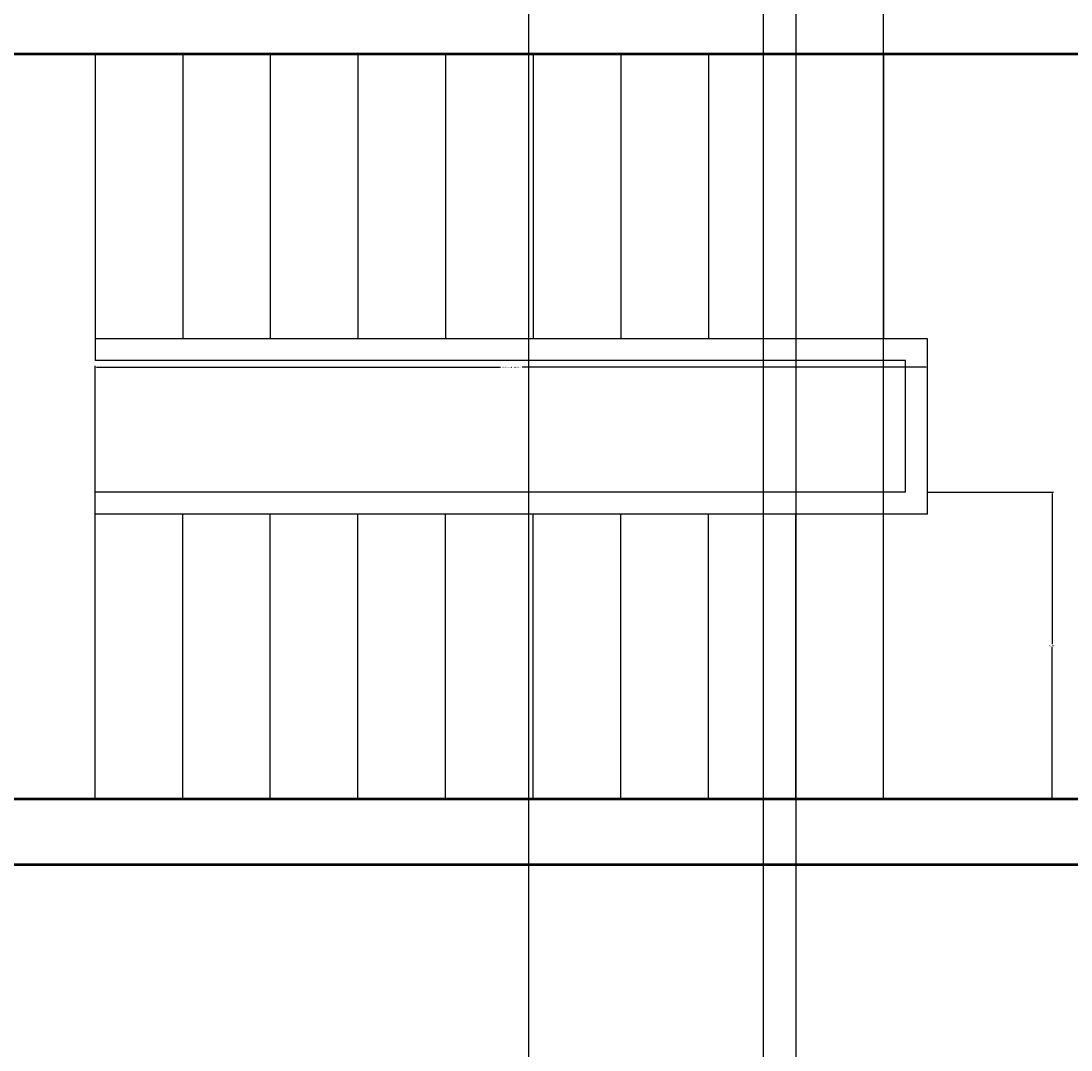
# Model space of a CAD drawing. Units: inches. Extents: x 5375 to 6084, y 16106 to 17259.
# Tile 13 of 32: x 5844 to 5988, y 16377 to 16518. Entities that reach past the tile are written whole.
import ezdxf

# ---------------------------------------------------------------- set-up
doc = ezdxf.new("R2010")
doc.units = ezdxf.units.IN
for name, color, linetype, lineweight in [('A-ANNO-DIMS', 2, 'Continuous', 18), ('STAIRCASE', 7, 'Continuous', 25), ('WALL', 6, 'Continuous', 50)]:
    doc.layers.add(name, color=color, linetype=linetype, lineweight=lineweight)
doc.styles.get("Standard").update_dxf_attribs({"font": 'arial.ttf'})
doc.dimstyles.get("Standard").update_dxf_attribs({"dimtxt": 0.18, "dimasz": 0.18, "dimexe": 0.18, "dimexo": 0.0625, "dimgap": 0.09, "dimtad": 0, "dimtih": 1, "dimtoh": 1, "dimdec": 4, "dimzin": 0, "dimdsep": 46, "dimtxsty": 'Standard', "dimcen": 0.09, "dimadec": 0, "dimazin": 0, "dimtfac": 1, "dimtdec": 4, "dimtofl": 0, "dimtmove": 0, "dimatfit": 3, "dimfxl": 1, "dimtolj": 1, "dimtzin": 0, "dimarcsym": 0})

# ---------------------------------------------------------------- blocks, each defined once
blk = doc.blocks.new('STAIR-FLIGHT-12IN-GOING')
for p, q in [((0, 42), (0, 0)), ((12, 42), (12, 3)), ((12, 42), (12, 3)), ((24, 42), (24, 3)), ((36, 42), (36, 3)), ((48, 42), (48, 3)), ((60, 42), (60, 3)), ((72, 42), (72, 3)), ((84, 42), (84, 3)), ((96, 42), (96, 3)), ((108, 42), (108, 3)), ((114, 3), (0, 3)), ((111, 0), (0, 0))]:
    blk.add_line(p, q)
blk = doc.blocks.new('*D24')
at = {"layer": 'A-ANNO-DIMS', "color": 0, "lineweight": -2, "transparency": 16777216}
for p, q in [((5854.62, 16453.64), (5854.62, 16470.86)), ((5854.8, 16470.68), (5910.14, 16470.68)), ((5968.44, 16470.68), (5913.1, 16470.68)), ((5968.62, 16453.64), (5968.62, 16470.86))]:
    blk.add_line(p, q, dxfattribs=at)
at = {"layer": 'A-ANNO-DIMS', "color": 0, "transparency": 16777216}
for points in [[(5854.8, 16470.71), (5854.8, 16470.65), (5854.62, 16470.68)], [(5968.44, 16470.71), (5968.44, 16470.65), (5968.62, 16470.68)]]:
    blk.add_solid(points, dxfattribs=at)
at = {"layer": 'Defpoints', "color": 0, "transparency": 16777216}
for p in [(5968.62, 16470.68), (5854.62, 16453.58), (5968.62, 16453.58)]:
    blk.add_point(p, dxfattribs=at)
at = {"layer": 'A-ANNO-DIMS', "color": 0, "transparency": 16777216, "insert": (5911.62, 16470.68), "char_height": 0.18, "attachment_point": 5}
blk.add_mtext('\\A1;STAIR FLIGHT 114 TYP.', dxfattribs=at)
blk = doc.blocks.new('*D25')
at = {"layer": 'A-ANNO-DIMS', "color": 0, "lineweight": -2, "transparency": 16777216}
for p, q in [((5968.68, 16453.58), (5985.9, 16453.58)), ((5985.72, 16453.4), (5985.72, 16432.76)), ((5985.72, 16411.76), (5985.72, 16432.4)), ((5968.68, 16411.58), (5985.9, 16411.58))]:
    blk.add_line(p, q, dxfattribs=at)
at = {"layer": 'A-ANNO-DIMS', "color": 0, "transparency": 16777216}
for points in [[(5985.69, 16453.4), (5985.75, 16453.4), (5985.72, 16453.58)], [(5985.69, 16411.76), (5985.75, 16411.76), (5985.72, 16411.58)]]:
    blk.add_solid(points, dxfattribs=at)
at = {"layer": 'Defpoints', "color": 0, "transparency": 16777216}
for p in [(5968.62, 16453.58), (5968.62, 16411.58), (5985.72, 16411.58)]:
    blk.add_point(p, dxfattribs=at)
at = {"layer": 'A-ANNO-DIMS', "color": 0, "transparency": 16777216, "insert": (5985.72, 16432.58), "char_height": 0.18, "attachment_point": 5}
blk.add_mtext('\\A1;42 TYP.', dxfattribs=at)
blk = doc.blocks.new('*D44')
at = {"layer": 'A-ANNO-DIMS', "color": 0, "lineweight": -2, "transparency": 16777216}
for p, q in [((5914, 16886.53), (5914, 16106.48)), ((5946.12, 16886.53), (5946.12, 16106.48)), ((5914.18, 16106.66), (5929.6, 16106.66)), ((5945.94, 16106.66), (5930.53, 16106.66))]:
    blk.add_line(p, q, dxfattribs=at)
at = {"layer": 'A-ANNO-DIMS', "color": 0, "transparency": 16777216}
for points in [[(5914.18, 16106.69), (5914.18, 16106.63), (5914, 16106.66)], [(5945.94, 16106.69), (5945.94, 16106.63), (5946.12, 16106.66)]]:
    blk.add_solid(points, dxfattribs=at)
at = {"layer": 'Defpoints', "color": 0, "transparency": 16777216}
for p in [(5914, 16886.6), (5946.12, 16886.6), (5914, 16106.66)]:
    blk.add_point(p, dxfattribs=at)
at = {"layer": 'A-ANNO-DIMS', "color": 0, "transparency": 16777216, "insert": (5930.06, 16106.66), "char_height": 0.18, "attachment_point": 5}
blk.add_mtext('\\A1;32.117', dxfattribs=at)
blk = doc.blocks.new('*D46')
at = {"layer": 'A-ANNO-DIMS', "color": 0, "lineweight": -2, "transparency": 16777216}
for p, q in [((5946.12, 16771.52), (5946.12, 16106.48)), ((5950.62, 16771.52), (5950.62, 16106.48)), ((5946.3, 16106.66), (5948.11, 16106.66)), ((5950.44, 16106.66), (5948.63, 16106.66))]:
    blk.add_line(p, q, dxfattribs=at)
at = {"layer": 'A-ANNO-DIMS', "color": 0, "transparency": 16777216}
for points in [[(5946.3, 16106.69), (5946.3, 16106.63), (5946.12, 16106.66)], [(5950.44, 16106.69), (5950.44, 16106.63), (5950.62, 16106.66)]]:
    blk.add_solid(points, dxfattribs=at)
at = {"layer": 'Defpoints', "color": 0, "transparency": 16777216}
for p in [(5946.12, 16771.58), (5950.62, 16771.58), (5950.62, 16106.66)]:
    blk.add_point(p, dxfattribs=at)
at = {"layer": 'A-ANNO-DIMS', "color": 0, "transparency": 16777216, "insert": (5948.37, 16106.66), "char_height": 0.18, "attachment_point": 5}
blk.add_mtext('\\A1;4.5', dxfattribs=at)
blk = doc.blocks.new('*D48')
at = {"layer": 'A-ANNO-DIMS', "color": 0, "lineweight": -2, "transparency": 16777216}
for p, q in [((5962.62, 16411.64), (5962.62, 17259.16)), ((5962.8, 17258.98), (5992.4, 17258.98)), ((6022.44, 17258.98), (5992.84, 17258.98)), ((6022.62, 16411.64), (6022.62, 17259.16))]:
    blk.add_line(p, q, dxfattribs=at)
at = {"layer": 'A-ANNO-DIMS', "color": 0, "transparency": 16777216}
for points in [[(5962.8, 17259.01), (5962.8, 17258.95), (5962.62, 17258.98)], [(6022.44, 17259.01), (6022.44, 17258.95), (6022.62, 17258.98)]]:
    blk.add_solid(points, dxfattribs=at)
at = {"layer": 'Defpoints', "color": 0, "transparency": 16777216}
for p in [(6022.62, 17258.98), (5962.62, 16411.58), (6022.62, 16411.58)]:
    blk.add_point(p, dxfattribs=at)
at = {"layer": 'A-ANNO-DIMS', "color": 0, "transparency": 16777216, "insert": (5992.62, 17258.98), "char_height": 0.18, "attachment_point": 5}
blk.add_mtext('\\A1;60', dxfattribs=at)

msp = doc.modelspace()

# ---------------------------------------------------------------- linework, layer by layer
at = {"layer": 'STAIRCASE'}
for p, q in [((5968.6199, 16450.5793), (5968.6199, 16474.5793)), ((5965.6199, 16453.5793), (5965.6199, 16471.5793))]:
    msp.add_line(p, q, dxfattribs=at)
at = {"layer": 'WALL'}
for p, q in [((5791.6199, 16513.5793), (6022.6199, 16513.5793)), ((5761.6199, 16411.5793), (6022.6199, 16411.5793)), ((5761.6199, 16402.5793), (6031.6199, 16402.5793))]:
    msp.add_line(p, q, dxfattribs=at)

# ---------------------------------------------------------------- block references
at = {"layer": 'STAIRCASE'}
msp.add_blockref('STAIR-FLIGHT-12IN-GOING', (5854.62, 16471.579), dxfattribs=at)
at = {"layer": 'STAIRCASE', "extrusion": (0, 0, -1), "zscale": -1, "rotation": 180}
msp.add_blockref('STAIR-FLIGHT-12IN-GOING', (-5854.62, 16453.5797), dxfattribs=at)

# ---------------------------------------------------------------- dimensions: what is measured, and where the dimension line sits
at = {"layer": 'A-ANNO-DIMS'}
for base, p1, p2, override, picture, middle in [((6022.6199, 17258.9793), (5962.6199, 16411.5793), (6022.6199, 16411.5793), {"dimdec": 0, "dimlfac": 1, "dimrnd": 0, "dimzin": 0, "dimdsep": 46, "dimlunit": 2}, '*D48', (5992.6199, 17258.9793)), ((5914.0033, 16106.6631), (5946.1199, 16886.5956), (5914.0033, 16886.5956), {"dimdec": 3, "dimlfac": 1, "dimrnd": 0, "dimzin": 0, "dimdsep": 46, "dimlunit": 2}, '*D44', (5930.0616, 16106.6631)), ((5950.6199, 16106.6631), (5946.1199, 16771.5793), (5950.6199, 16771.5793), {"dimdec": 1, "dimlfac": 1, "dimrnd": 0, "dimzin": 0, "dimdsep": 46, "dimlunit": 2}, '*D46', (5948.3699, 16106.6631))]:
    dim = msp.add_linear_dim(base=base, p1=p1, p2=p2, dimstyle='Standard', override=override, dxfattribs=at)
    dim.commit()
    dim.dimension.update_dxf_attribs({"geometry": picture, "text_midpoint": middle})
dim = msp.add_linear_dim(base=(5968.6199, 16470.6793), p1=(5854.6199, 16453.5793), p2=(5968.6199, 16453.5793), text='STAIR FLIGHT <> TYP.', dimstyle='Standard', override={"dimdec": 0, "dimlfac": 1, "dimrnd": 0, "dimzin": 0, "dimdsep": 46, "dimlunit": 2}, dxfattribs=at)
dim.commit()
dim.dimension.update_dxf_attribs({"geometry": '*D24', "text_midpoint": (5911.6199, 16470.6793)})
dim = msp.add_linear_dim(base=(5985.7199, 16411.5793), p1=(5968.6199, 16453.5793), p2=(5968.6199, 16411.5793), angle=270, text='<> TYP.', dimstyle='Standard', override={"dimdec": 0, "dimlfac": 1, "dimrnd": 0, "dimzin": 0, "dimdsep": 46, "dimlunit": 2}, dxfattribs=at)
dim.commit()
dim.dimension.update_dxf_attribs({"geometry": '*D25', "text_midpoint": (5985.7199, 16432.5793)})

doc.saveas('drawing.dxf')
